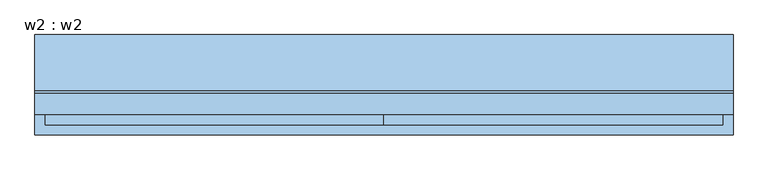
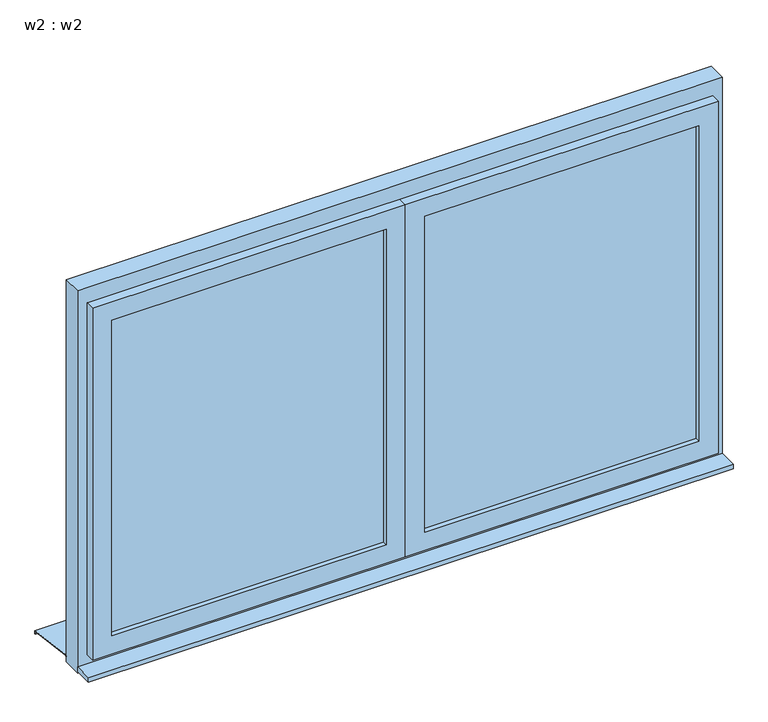
"""IFC4 building model written with IfcOpenShell, lengths in millimetres: window geometry, w2 : w2."""

from ifc_helpers import new_model, si_unit, frame, origin, place, context, project, spatial, polyline, outline, extrude, faceted_brep, source, transform, mapped, element, save


def w2_w2_7b90d420(model_context):
    return source(origin(), model_context, "Body", "SolidModel", [
        extrude(outline(polyline([(-15.6778457, 1020.0), (144.3, 1000.0), (144.3, 990.0), (142.3, 990.0), (142.3, 998.3604634), (-15.8759277, 1018.0), (-25.7, 1018.0), (-25.7, 1020.0), (-15.6778457, 1020.0)])), frame((-1005.0, 0.0, 0.0), z_axis=(1.0, 0.0, 0.0), x_axis=(0.0, 1.0, 0.0)), (0.0, 0.0, 1.0), 2010.0),
        extrude(outline(polyline([(-1005.0, -144.3), (-1005.0, -85.7), (1005.0, -85.7), (1005.0, -144.3), (-1005.0, -144.3)])), frame((0.0, 0.0, 1005.0), z_axis=(0.0, 0.0, 1.0), x_axis=(1.0, 0.0, 0.0)), (0.0, 0.0, 1.0), 15.0),
        extrude(outline(polyline([(60.0, -70.7), (915.0, -70.7), (915.0, -100.7), (60.0, -100.7), (60.0, -70.7)])), frame((0.0, 0.0, 1110.0), z_axis=(0.0, 0.0, 1.0), x_axis=(1.0, 0.0, 0.0)), (0.0, 0.0, 1.0), 1040.0),
        extrude(outline(polyline([(-915.0, -70.7), (-60.0, -70.7), (-60.0, -100.7), (-915.0, -100.7), (-915.0, -70.7)])), frame((0.0, 0.0, 1110.0), z_axis=(0.0, 0.0, 1.0), x_axis=(1.0, 0.0, 0.0)), (0.0, 0.0, 1.0), 1040.0),
        extrude(outline(polyline([(2260.0, -1005.0), (1000.0, -1005.0), (1000.0, 1005.0), (2260.0, 1005.0), (2260.0, -1005.0)]), holes=[polyline([(2180.0, -945.0), (2180.0, 945.0), (1080.0, 945.0), (1080.0, -945.0), (2180.0, -945.0)])]), frame((0.0, -85.7, 0.0), z_axis=(0.0, 1.0, 0.0), x_axis=(0.0, 0.0, 1.0)), (0.0, 0.0, 1.0), 60.0),
        extrude(outline(polyline([(30.0, -85.7), (-30.0, -85.7), (-30.0, -25.7), (30.0, -25.7), (30.0, -85.7)])), frame((0.0, 0.0, 1080.0), z_axis=(0.0, 0.0, 1.0), x_axis=(1.0, 0.0, 0.0)), (0.0, 0.0, 1.0), 1100.0),
        faceted_brep([(30.0, -85.7, 1080.0), (30.0, -55.7, 1080.0), (945.0, -55.7, 1080.0), (945.0, -85.7, 1080.0), (945.0, -55.7, 2180.0), (945.0, -85.7, 2180.0), (30.0, -55.7, 2180.0), (915.0, -55.7, 2150.0), (60.0, -55.7, 2150.0), (60.0, -55.7, 1110.0), (915.0, -55.7, 1110.0), (975.0, -85.7, 1050.0), (0.0, -85.7, 1050.0), (0.0, -85.7, 2210.0), (975.0, -85.7, 2210.0), (30.0, -85.7, 2180.0), (0.0, -115.7, 1050.0), (975.0, -115.7, 1050.0), (975.0, -115.7, 2210.0), (0.0, -115.7, 2210.0), (915.0, -115.7, 1110.0), (60.0, -115.7, 1110.0), (60.0, -115.7, 2150.0), (915.0, -115.7, 2150.0)], [[[0, 1, 2, 3]], [[3, 2, 4, 5]], [[2, 1, 6, 4], [7, 8, 9, 10]], [[11, 12, 13, 14], [5, 15, 0, 3]], [[16, 12, 11, 17]], [[17, 11, 14, 18]], [[18, 19, 16, 17], [20, 21, 22, 23]], [[9, 21, 20, 10]], [[10, 20, 23, 7]], [[15, 6, 1, 0]], [[19, 13, 12, 16]], [[8, 22, 21, 9]], [[5, 4, 6, 15]], [[18, 14, 13, 19]], [[7, 23, 22, 8]]]),
        faceted_brep([(-945.0, -85.7, 1080.0), (-945.0, -55.7, 1080.0), (-30.0, -55.7, 1080.0), (-30.0, -85.7, 1080.0), (-30.0, -55.7, 2180.0), (-30.0, -85.7, 2180.0), (-945.0, -55.7, 2180.0), (-60.0, -55.7, 2150.0), (-915.0, -55.7, 2150.0), (-915.0, -55.7, 1110.0), (-60.0, -55.7, 1110.0), (0.0, -85.7, 1050.0), (-975.0, -85.7, 1050.0), (-975.0, -85.7, 2210.0), (0.0, -85.7, 2210.0), (-945.0, -85.7, 2180.0), (-975.0, -115.7, 1050.0), (0.0, -115.7, 1050.0), (0.0, -115.7, 2210.0), (-975.0, -115.7, 2210.0), (-60.0, -115.7, 1110.0), (-915.0, -115.7, 1110.0), (-915.0, -115.7, 2150.0), (-60.0, -115.7, 2150.0)], [[[0, 1, 2, 3]], [[3, 2, 4, 5]], [[2, 1, 6, 4], [7, 8, 9, 10]], [[11, 12, 13, 14], [5, 15, 0, 3]], [[16, 12, 11, 17]], [[17, 11, 14, 18]], [[18, 19, 16, 17], [20, 21, 22, 23]], [[9, 21, 20, 10]], [[10, 20, 23, 7]], [[15, 6, 1, 0]], [[19, 13, 12, 16]], [[8, 22, 21, 9]], [[5, 4, 6, 15]], [[18, 14, 13, 19]], [[7, 23, 22, 8]]]),
    ])


if __name__ == "__main__":
    model = new_model("IFC4")
    model_context = context("Model", 3, world=origin())
    ifc_project = project(units=[si_unit("LENGTHUNIT", "METRE", prefix="MILLI")], contexts=[model_context])
    site = spatial("IfcSite", under=ifc_project)
    building = spatial("IfcBuilding", under=site)
    placement = place(None, origin())
    w2_w2_shape = w2_w2_7b90d420(model_context)
    element("IfcWindow", 1, ObjectType="w2 : w2", at=placement, inside=building, context=model_context, shape_type="MappedRepresentation", body=[
        mapped(w2_w2_shape, transform((0.0, 0.0, 0.0), x_axis=(1.0, 0.0, 0.0), y_axis=(0.0, 1.0, 0.0), z_axis=(0.0, 0.0, 1.0))),
    ])
    save(model, "model.ifc")

# Revit data of these elements
# Type "w2 : w2"
#   Type Mark = "18"
#   Operation = "DoublePanelVertical"
#   Keynote = "16.05.01"
#   Analytic Construction = "<None>"
#   Rough Width = 6' - 7.13386"
#   Rough Height = 4' - 1.6063"
#   Rahmentiefe = 0' - 2.3622"
#   Rahmenhöhe unten = 0' - 3.14961"
#   Rahmehöhe oben = 0' - 3.14961"
#   Rahmenbreite = 0' - 2.3622"
#   Heat Transfer Coefficient (U) = 2.81836 BTU/(h·ft²·°F)
#   Height = 4' - 1.6063"
#   Flügeltiefe = 0' - 2.3622"
#   Flügelbreite = 0' - 2.3622"
#   Einbautiefe (von außen) [instance default] = 0' - 5.51181"
#   Width = 6' - 7.13386"
#   Kippflügel [instance default] = yes
#   Drehflügel im Grundriß darstellen [instance default] = no
#   Drehflügel [instance default] = yes
#   Define Thermal Properties by = 1
#   Rahmen [instance default] = none
#   Glas [instance default] = blue glass
#   Flügel [instance default] = WINDOW COLOUR WHITE
#   Fensterbank aussen [instance default] = WINDOW COLOUR WHITE
#   Fensterbank innen [instance default] = WINDOW COLOUR WHITE
#   Visual Light Transmittance = 0
#   Thermal Resistance (R) = 0
#   Solar Heat Gain Coefficient = 0
#   Wall Closure = (empty or 0)
# Element 1 (IfcWindow, "w2 : w2")
#   Materials on its faces: "WINDOW COLOUR WHITE", "blue glass"
# Materials
#   "blue glass": class "System", colour RGB 0 0 255, transparency 0.75, Cost = 0
#   "WINDOW COLOUR WHITE": class "Generic", colour RGB 120 120 120, transparency 0, Cost = 0
